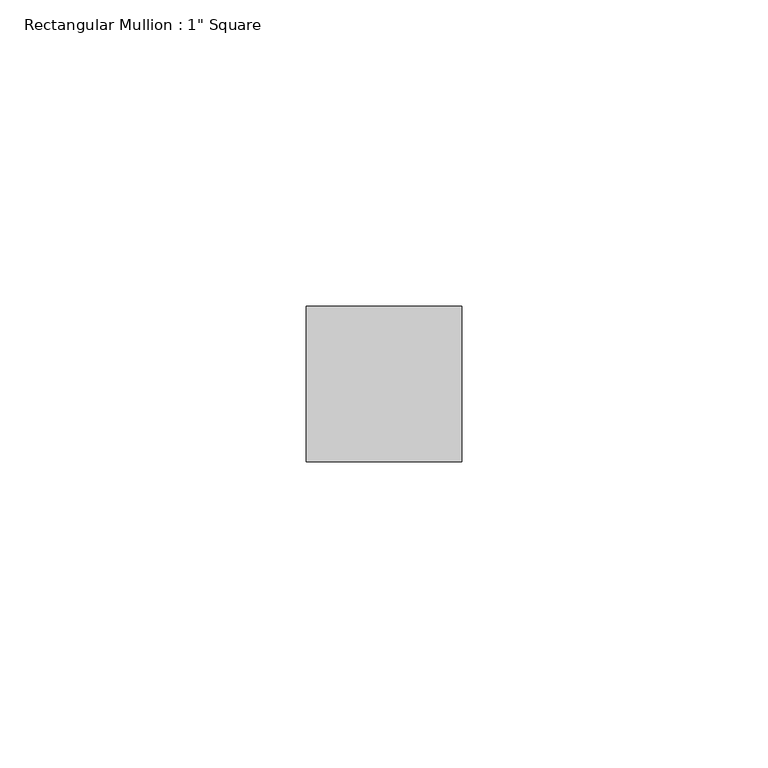
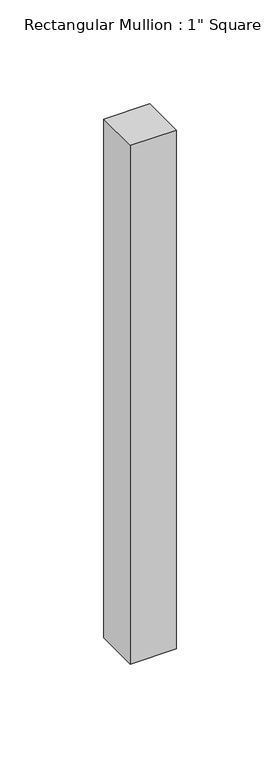
"""IFC4 building model written with IfcOpenShell, lengths in millimetres: member geometry."""

from ifc_helpers import new_model, si_unit, frame, origin, place, context, project, spatial, polyline, outline, extrude, source, transform, mapped, element, save


def member_d020295e(model_context):
    return source(origin(), model_context, "Body", "SweptSolid", [
        extrude(outline(polyline([(12.7, 12.7), (12.7, -12.7), (-12.7, -12.7), (-12.7, 12.7), (12.7, 12.7)])), frame((0.0, 0.0, -304.8), z_axis=(0.0, 0.0, 1.0), x_axis=(1.0, 0.0, 0.0)), (0.0, 0.0, 1.0), 304.8),
    ])


if __name__ == "__main__":
    model = new_model("IFC4")
    model_context = context("Model", 3, world=origin())
    ifc_project = project(units=[si_unit("LENGTHUNIT", "METRE", prefix="MILLI")], contexts=[model_context])
    site = spatial("IfcSite", under=ifc_project)
    building = spatial("IfcBuilding", under=site)
    placement = place(None, origin())
    member_shape = member_d020295e(model_context)
    element("IfcMember", 1, ObjectType="Rectangular Mullion : 1\" Square", at=placement, inside=building, context=model_context, shape_type="MappedRepresentation", body=[
        mapped(member_shape, transform((0.0, 0.0, 0.0), x_axis=(1.0, 0.0, 0.0), y_axis=(0.0, 1.0, 0.0), z_axis=(0.0, 0.0, 1.0))),
    ])
    save(model, "model.ifc")

# Revit data of these elements
# Type "Rectangular Mullion : 1\" Square"
#   built-in parameter 1007304 = 0.0833333 (stored number, unit not read)
#   built-in parameter 1007301 = 0.0416667 (stored number, unit not read)
#   built-in parameter 1007300 = 0.0416667 (stored number, unit not read)
